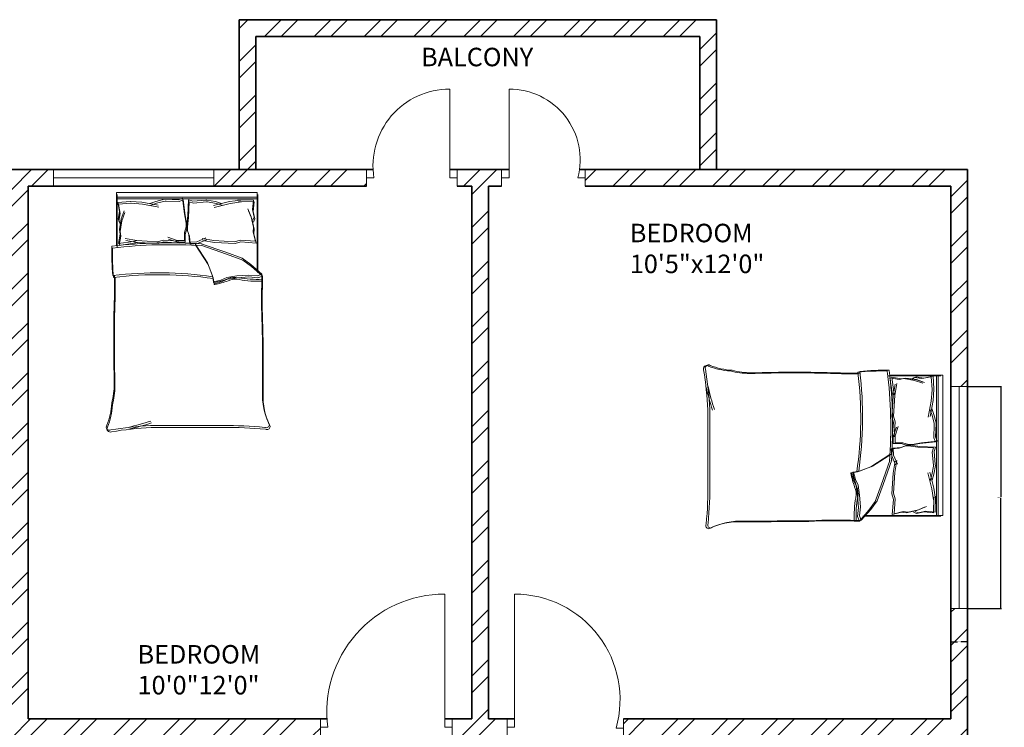
# Model space of a CAD drawing. Units: inches. Extents: x 1944 to 3454, y 1352 to 3055.
# Tile 9 of 17: x 2314 to 2580, y 2031 to 2223. Entities that reach past the tile are written whole.
import ezdxf

# ---------------------------------------------------------------- set-up
doc = ezdxf.new("R2010")
doc.units = ezdxf.units.IN
for name, color, linetype, lineweight in [('A-ANNO-DIMS', 2, 'Continuous', 18), ('A-AREA-IDEN', 7, 'Continuous', 18), ('A-DOOR', 3, 'Continuous', 20), ('A-FURN', 8, 'Continuous', 13), ('A-GLAZ', 4, 'Continuous', 18), ('A-WALL', 7, 'Continuous', 35), ('A-WALL-PATT', 252, 'Continuous', 13)]:
    doc.layers.add(name, color=color, linetype=linetype, lineweight=lineweight)
doc.styles.get("Standard").update_dxf_attribs({"font": 'arial.ttf'})
doc.dimstyles.get("Standard").update_dxf_attribs({"dimtxt": 0.18, "dimasz": 0.18, "dimexe": 0.18, "dimexo": 0.0625, "dimgap": 0.09, "dimtad": 0, "dimtih": 1, "dimtoh": 1, "dimdec": 4, "dimzin": 0, "dimdsep": 46, "dimtxsty": 'Standard', "dimcen": 0.09, "dimadec": 0, "dimazin": 0, "dimtfac": 1, "dimtdec": 4, "dimtofl": 0, "dimtmove": 0, "dimatfit": 3, "dimfxl": 1, "dimtolj": 1, "dimtzin": 0, "dimarcsym": 0})

# ---------------------------------------------------------------- blocks, each defined once
blk = doc.blocks.new('BED-WITH-PILLOWS-01')
for p, q in [((0, 40.75), (21.15, 40.75)), ((0, 40.75), (21.15, 40.75)), ((0, 2.76), (0, 40.75)), ((0.51, 40.93), (21.66, 40.93)), ((0.51, 40.93), (21.66, 40.93)), ((1.22, 2.76), (1.22, 40.75)), ((1.22, 2.76), (1.22, 40.75)), ((1.73, 2.94), (1.73, 40.93)), ((1.73, 2.94), (1.73, 40.93)), ((2.54, 40.01), (2.46, 35.72)), ((2.54, 40.01), (2.46, 35.72)), ((2.54, 40.01), (5.09, 39.71)), ((2.54, 40.01), (5.09, 39.71)), ((4.58, 39.53), (6.63, 40.01)), ((4.58, 39.53), (6.63, 40.01)), ((5.09, 39.71), (7.14, 40.19)), ((5.09, 39.71), (7.14, 40.19)), ((6.63, 40.01), (7.46, 39.6)), ((6.63, 40.01), (7.46, 39.6)), ((9.91, 40.01), (7.07, 39.38)), ((9.91, 40.01), (7.07, 39.38)), ((7.14, 40.19), (7.97, 39.78)), ((7.14, 40.19), (7.97, 39.78)), ((11.19, 39.86), (9.91, 40.01)), ((11.19, 39.86), (9.91, 40.01)), ((13.17, 40.3), (10.68, 39.68)), ((13.17, 40.3), (10.68, 39.68)), ((13.68, 40.48), (11.19, 39.86)), ((13.68, 40.48), (11.19, 39.86)), ((12.85, 36.22), (13.17, 40.3)), ((12.85, 36.22), (13.17, 40.3)), ((13.36, 36.4), (13.68, 40.48)), ((13.36, 36.4), (13.68, 40.48)), ((22.05, 42.02), (19.47, 39.08)), ((22.05, 42.02), (19.47, 39.08)), ((22.56, 42.21), (19.98, 39.26)), ((22.56, 42.21), (19.98, 39.26)), ((23.44, 42.09), (22.05, 42.02, 3.08)), ((23.44, 42.09), (22.05, 42.02, 3.08)), ((22.55, 40.8), (22.05, 42.02)), ((22.55, 40.8), (22.05, 42.02)), ((22.3, 38.34), (22.55, 40.8)), ((22.3, 38.34), (22.55, 40.8)), ((23.95, 42.27), (22.56, 42.21, 3.08)), ((23.95, 42.27), (22.56, 42.21, 3.08)), ((23.05, 40.98), (22.56, 42.21)), ((23.05, 40.98), (22.56, 42.21)), ((22.81, 38.52), (23.05, 40.98)), ((22.81, 38.52), (23.05, 40.98)), ((2.03, 39.83), (1.96, 35.54)), ((2.03, 39.83), (1.96, 35.54)), ((2.03, 39.83), (4.58, 39.53)), ((2.03, 39.83), (4.58, 39.53)), ((6.56, 39.2), (4.43, 38.26)), ((6.56, 39.2), (4.43, 38.26)), ((7.07, 39.38), (4.94, 38.44)), ((7.07, 39.38), (4.94, 38.44)), ((9.4, 39.83), (6.56, 39.2)), ((9.4, 39.83), (6.56, 39.2)), ((10.68, 39.68), (9.4, 39.83)), ((10.68, 39.68), (9.4, 39.83)), ((19.47, 39.08), (17.75, 36.74)), ((19.47, 39.08), (17.75, 36.74)), ((19.98, 39.26), (18.26, 36.92)), ((19.98, 39.26), (18.26, 36.92)), ((22.55, 35.26), (22.3, 38.34)), ((22.55, 35.26), (22.3, 38.34)), ((23.05, 35.44), (22.81, 38.52)), ((23.05, 35.44), (22.81, 38.52)), ((1.96, 35.54), (2.02, 36.34)), ((1.96, 35.54), (2.02, 36.34)), ((2.02, 36.34), (2.44, 33.32)), ((2.02, 36.34), (2.44, 33.32)), ((2.46, 35.72), (2.53, 36.52)), ((2.46, 35.72), (2.53, 36.52)), ((2.53, 36.52), (2.95, 33.5)), ((2.53, 36.52), (2.95, 33.5)), ((13.3, 34.66), (12.85, 36.22)), ((13.3, 34.66), (12.85, 36.22)), ((12.95, 29.09), (13.3, 34.66)), ((12.95, 29.09), (13.3, 34.66)), ((13.8, 34.84), (13.36, 36.4)), ((13.8, 34.84), (13.36, 36.4)), ((13.46, 29.27), (13.8, 34.84)), ((13.46, 29.27), (13.8, 34.84)), ((17.75, 36.74), (16.15, 32.31)), ((17.75, 36.74), (16.15, 32.31)), ((18.26, 36.92), (16.66, 32.49)), ((18.26, 36.92), (16.66, 32.49)), ((22.92, 32.55), (22.55, 35.26)), ((22.92, 32.55), (22.55, 35.26)), ((23.42, 32.74), (23.05, 35.44)), ((23.42, 32.74), (23.05, 35.44)), ((2.44, 33.32), (3.51, 29.01)), ((2.44, 33.32), (3.51, 29.01)), ((2.95, 33.5), (4.02, 29.19)), ((2.95, 33.5), (4.02, 29.19)), ((16.15, 32.31), (13.82, 25.68)), ((16.15, 32.31), (13.82, 25.68)), ((16.66, 32.49), (14.33, 25.86)), ((16.66, 32.49), (14.33, 25.86)), ((23.65, 30.95), (22.92, 32.55)), ((23.65, 30.95), (22.92, 32.55)), ((24.16, 31.13), (23.42, 32.74)), ((24.16, 31.13), (23.42, 32.74)), ((2.45, 29.52), (2.02, 27.19)), ((2.45, 29.52), (2.02, 27.19)), ((2.92, 31.16), (2.45, 29.52)), ((2.92, 31.16), (2.45, 29.52)), ((2.95, 29.7), (2.52, 27.37)), ((2.95, 29.7), (2.52, 27.37)), ((3.43, 31.34), (2.95, 29.7)), ((3.43, 31.34), (2.95, 29.7)), ((24.15, 28.98), (23.65, 30.95)), ((24.15, 28.98), (23.65, 30.95)), ((24.65, 29.17), (24.16, 31.13)), ((24.65, 29.16), (24.16, 31.13)), ((62.99, 11.97), (62.99, 31.54)), ((62.99, 11.97), (62.99, 31.54)), ((63.5, 12.16), (63.5, 31.72)), ((63.5, 12.15), (63.5, 31.72)), ((2.02, 27.19), (2.03, 26.93)), ((2.02, 27.19), (2.03, 26.93)), ((2.03, 26.93), (2.37, 23.41)), ((2.03, 26.93), (2.37, 23.41)), ((2.52, 27.37), (2.54, 27.12)), ((2.52, 27.37), (2.54, 27.11)), ((2.54, 27.12), (2.88, 23.6)), ((2.54, 27.11), (2.88, 23.6)), ((13.31, 24.44), (12.28, 26.88)), ((13.31, 24.44), (12.28, 26.88)), ((12.42, 25.88), (12.95, 29.09)), ((12.42, 25.88), (12.95, 29.09)), ((13.81, 24.62), (12.79, 27.07)), ((13.81, 24.62), (12.79, 27.06)), ((12.93, 26.07), (13.46, 29.27)), ((12.93, 26.07), (13.46, 29.27)), ((13.82, 24.05), (18.98, 27.38)), ((13.82, 24.05), (18.98, 27.38)), ((14.33, 24.23), (19.49, 27.56)), ((14.33, 24.23), (19.49, 27.56)), ((18.98, 27.38), (22.55, 28.74)), ((18.98, 27.38), (22.55, 28.74)), ((19.49, 27.56), (23.05, 28.92)), ((19.49, 27.56), (23.05, 28.92)), ((22.55, 28.74), (24.15, 28.98)), ((22.55, 28.74), (24.15, 28.98)), ((23.05, 28.92), (24.65, 29.17)), ((23.05, 28.92), (24.65, 29.16)), ((13.43, 22.49), (13.31, 24.44)), ((13.43, 22.49), (13.31, 24.44)), ((13.94, 22.67), (13.81, 24.62)), ((13.94, 22.67), (13.81, 24.62)), ((2.37, 23.41), (1.98, 22.24)), ((2.37, 23.41), (1.98, 22.24)), ((1.98, 22.24), (6.25, 22.04)), ((1.98, 22.24), (6.25, 22.04)), ((2.88, 23.6), (2.49, 22.42)), ((2.88, 23.6), (2.49, 22.42)), ((2.49, 22.42), (6.76, 22.23)), ((2.49, 22.42), (6.76, 22.23)), ((5.74, 21.11), (8.27, 21.57)), ((5.74, 21.11), (8.27, 21.57)), ((6.25, 22.04), (8.81, 21.74)), ((6.25, 22.04), (8.81, 21.74)), ((6.25, 21.29), (8.78, 21.75)), ((6.25, 21.29), (8.78, 21.75)), ((6.76, 22.23), (9.31, 21.93)), ((6.76, 22.23), (9.31, 21.93)), ((8.27, 21.57), (9.3, 21.57)), ((8.27, 21.57), (9.3, 21.57)), ((8.78, 21.75), (9.81, 21.75)), ((8.78, 21.75), (9.81, 21.75)), ((8.81, 21.74), (9.84, 21.81)), ((8.81, 21.74), (9.84, 21.81)), ((9.3, 21.57), (10.8, 21.11)), ((9.3, 21.57), (10.8, 21.11)), ((9.31, 21.93), (10.35, 21.99)), ((9.31, 21.93), (10.35, 21.99)), ((9.81, 21.75), (11.3, 21.29)), ((9.81, 21.75), (11.3, 21.29)), ((9.84, 21.81), (11.3, 22.36)), ((9.84, 21.81), (11.3, 22.36)), ((10.35, 21.99), (11.81, 22.54)), ((10.35, 21.99), (11.81, 22.54)), ((11.3, 22.36), (13.43, 22.49)), ((11.3, 22.36), (13.43, 22.49)), ((11.81, 22.54), (13.94, 22.67)), ((11.81, 22.54), (13.94, 22.67)), ((1.49, 20.65), (5.74, 21.11)), ((1.49, 20.65), (5.74, 21.11)), ((1.95, 19.5), (1.49, 20.65)), ((1.95, 19.5), (1.49, 20.65)), ((1.83, 15.97), (1.95, 19.5)), ((1.83, 15.97), (1.95, 19.5)), ((1.99, 20.83), (6.25, 21.29)), ((1.99, 20.83), (6.25, 21.29)), ((2.45, 19.69), (1.99, 20.83)), ((2.45, 19.69), (1.99, 20.83)), ((2.34, 16.15), (2.45, 19.69)), ((2.34, 16.15), (2.45, 19.69)), ((10.8, 21.11), (12.93, 21.11)), ((10.8, 21.11), (12.93, 21.11)), ((11.3, 21.29), (13.44, 21.29)), ((11.3, 21.29), (13.44, 21.29)), ((12.93, 19.16), (12.06, 16.66)), ((12.93, 19.16), (12.06, 16.66)), ((13.44, 19.34), (12.57, 16.84)), ((13.44, 19.34), (12.57, 16.84)), ((12.85, 15.41), (13.17, 19.49)), ((12.85, 15.41), (13.17, 19.49)), ((12.93, 21.11), (12.93, 19.16)), ((12.93, 21.11), (12.93, 19.16)), ((13.36, 15.59), (13.68, 19.67)), ((13.36, 15.59), (13.68, 19.67)), ((13.44, 21.29), (13.44, 19.34)), ((13.44, 21.29), (13.44, 19.34)), ((2.34, 15.9), (2.34, 16.15)), ((2.34, 15.9), (2.34, 16.15)), ((1.83, 15.71), (1.83, 15.97)), ((1.83, 15.71), (1.83, 15.97)), ((2.41, 13.42), (1.83, 15.71)), ((2.41, 13.42), (1.83, 15.71)), ((2.91, 13.6), (2.34, 15.9)), ((2.91, 13.6), (2.34, 15.9)), ((2.98, 11.81), (2.41, 13.42)), ((2.98, 11.81), (2.41, 13.42)), ((2.64, 9.62), (3.44, 13.99)), ((2.64, 9.62), (3.44, 13.99)), ((3.49, 11.99), (2.91, 13.6)), ((3.49, 11.99), (2.91, 13.6)), ((3.14, 9.81), (3.95, 14.17)), ((3.14, 9.81), (3.95, 14.17)), ((13.3, 13.85), (12.85, 15.41)), ((13.3, 13.85), (12.85, 15.41)), ((12.95, 8.28), (13.3, 13.85)), ((12.95, 8.28), (13.3, 13.85)), ((13.8, 14.03), (13.36, 15.59)), ((13.8, 14.03), (13.36, 15.59)), ((13.46, 8.46), (13.8, 14.03)), ((13.46, 8.46), (13.8, 14.03)), ((2.41, 6.59), (2.64, 9.62)), ((2.41, 6.59), (2.64, 9.62)), ((2.91, 6.77), (3.14, 9.81)), ((2.91, 6.77), (3.14, 9.81)), ((12.42, 5.07), (12.95, 8.28)), ((12.42, 5.07), (12.95, 8.28)), ((12.93, 5.25), (13.46, 8.46)), ((12.93, 5.25), (13.46, 8.46)), ((12.95, 8.28), (13.21, 7.38)), ((12.95, 8.28), (13.21, 7.38)), ((13.46, 8.46), (13.72, 7.56)), ((13.46, 8.46), (13.72, 7.56)), ((2.39, 6.5), (2.41, 6.59)), ((2.39, 6.5), (2.41, 6.59)), ((2.65, 3.1), (2.39, 6.5)), ((2.65, 3.1), (2.39, 6.5)), ((2.9, 6.68), (2.91, 6.77)), ((2.9, 6.68), (2.91, 6.77)), ((3.16, 3.28), (2.9, 6.68)), ((3.16, 3.28), (2.9, 6.68)), ((13.21, 7.38), (13.78, 3.33)), ((13.21, 7.38), (13.78, 3.33)), ((13.72, 7.56), (14.29, 3.51)), ((13.72, 7.56), (14.29, 3.51)), ((14.4, 2.76), (0, 2.76)), ((14.4, 2.76), (0, 2.76)), ((14.9, 2.94), (0.51, 2.94)), ((14.9, 2.94), (0.51, 2.94)), ((2.64, 3.1), (5.16, 3.56)), ((2.64, 3.1), (5.16, 3.56)), ((3.14, 3.28), (5.67, 3.74)), ((3.14, 3.28), (5.67, 3.74)), ((7.12, 4.02), (4.93, 4.82)), ((7.12, 4.01), (4.93, 4.82)), ((5.16, 3.56), (7.23, 3.21)), ((5.16, 3.56), (7.23, 3.21)), ((7.63, 4.2), (5.44, 5)), ((7.63, 4.2), (5.44, 5)), ((5.67, 3.74), (7.74, 3.39)), ((5.67, 3.74), (7.74, 3.39)), ((9.99, 3.56), (7.12, 4.02)), ((9.99, 3.56), (7.12, 4.01)), ((7.23, 3.21), (8.04, 3.67)), ((7.23, 3.21), (8.04, 3.67)), ((10.5, 3.74), (7.63, 4.2)), ((10.5, 3.74), (7.63, 4.2)), ((7.74, 3.39), (8.55, 3.85)), ((7.74, 3.39), (8.55, 3.85)), ((11.26, 3.79), (9.99, 3.56)), ((11.26, 3.79), (9.99, 3.56)), ((11.76, 3.97), (10.5, 3.74)), ((11.76, 3.97), (10.5, 3.74)), ((13.78, 3.33), (11.26, 3.79)), ((13.78, 3.33), (11.26, 3.79)), ((14.29, 3.51), (11.76, 3.97)), ((14.29, 3.51), (11.76, 3.97))]:
    blk.add_line(p, q)
for centre, radius, start, end in [((54.58, 60.54), 18.33, 267.4714, 296.4681), ((54.58, 60.54), 18.33, 267.4714, 296.4681), ((55.09, 60.72), 18.33, 267.4714, 296.4681), ((55.09, 60.72), 18.33, 267.4714, 296.4681), ((62.69, 43.25), 0.876, 332.6588, 86.02), ((62.69, 43.25), 0.876, 332.6588, 86.02), ((168.74, 32.71), 105.75, 174.4998, 180.6351), ((168.74, 32.71), 105.75, 174.4998, 180.6351), ((63.2, 43.43), 0.876, 332.6588, 86.02), ((63.2, 43.43), 0.876, 332.6588, 86.02), ((169.24, 32.89), 105.75, 174.4998, 180.6351), ((169.24, 32.89), 105.75, 174.4998, 180.6351), ((-5.29, 40.8), 28.76, 349.8763, 2.5657), ((-5.29, 40.8), 28.76, 349.8763, 2.5657), ((28.87, 144.88), 102.94, 266.9791, 273.8365), ((28.87, 144.88), 102.94, 266.9791, 273.8365), ((-4.78, 40.98), 28.76, 349.8763, 2.5657), ((-4.78, 40.98), 28.76, 349.8763, 2.5657), ((29.37, 145.06), 102.94, 266.9791, 273.8365), ((29.37, 145.06), 102.94, 266.9791, 273.8365), ((53.91, -3583.94), 3626.16, 90.00217, 90.28689), ((53.91, -3583.94), 3626.16, 90.00217, 90.28689), ((54.42, -3583.76), 3626.16, 90.00217, 90.28689), ((54.42, -3583.76), 3626.16, 90.00217, 90.28689), ((27.87, 34.77), 4.95, 168.6608, 203.7384), ((27.87, 34.77), 4.95, 168.6608, 203.7384), ((28.38, 34.95), 4.95, 168.6608, 203.7384), ((28.38, 34.95), 4.95, 168.6608, 203.7384), ((1.18, 24.76), 23.57, 10.6617, 19.8806), ((1.18, 24.76), 23.57, 10.6617, 19.8806), ((1.69, 24.95), 23.57, 10.6617, 19.8806), ((1.69, 24.94), 23.57, 10.6617, 19.8806), ((24.7, 29.3), 0.147, 250.2464, 1.1377), ((24.7, 29.3), 0.147, 250.2464, 1.1377), ((124.25, 14.11), 102.56, 171.7845, 186.9006), ((124.25, 14.11), 102.56, 171.7845, 186.9006), ((124.76, 14.3), 102.56, 171.7845, 186.9006), ((124.76, 14.3), 102.56, 171.7845, 186.9006), ((24.2, 29.12), 0.147, 250.2464, 1.1377), ((24.2, 29.12), 0.147, 250.2464, 1.1377), ((144.71, 16.98), 131.13, 176.0865, 186.7821), ((144.71, 16.98), 131.13, 176.0865, 186.7821), ((145.22, 17.16), 131.13, 176.0865, 186.7821), ((145.22, 17.16), 131.13, 176.0865, 186.7821), ((-18.85, -13.69), 84.62, 13.3832, 17.7053), ((-18.85, -13.69), 84.62, 13.3832, 17.7053), ((-18.34, -13.51), 84.62, 13.3832, 17.7053), ((-18.34, -13.51), 84.62, 13.3832, 17.7053), ((159.64, 17.03), 96.78, 182.9958, 189.4091), ((159.64, 17.03), 96.78, 182.9958, 189.4091), ((160.15, 17.21), 96.78, 182.9958, 189.4091), ((160.15, 17.21), 96.78, 182.9958, 189.4091), ((15.97, 67.69), 66.22, 268.7218, 275.604), ((15.97, 67.69), 66.22, 268.7218, 275.604), ((16.48, 67.88), 66.22, 268.7218, 275.604), ((16.48, 67.88), 66.22, 268.7218, 275.604), ((24.78, -132.99), 135.22, 88.4762, 91.0082), ((24.78, -132.99), 135.22, 88.4762, 91.0082), ((25.29, -132.81), 135.22, 88.4762, 91.0082), ((25.29, -132.81), 135.22, 88.4762, 91.0082), ((40.23, 385.38), 383.38, 268.2277, 271.7185), ((40.23, 385.38), 383.38, 268.2277, 271.7185), ((40.74, 385.56), 383.38, 268.2277, 271.7185), ((40.74, 385.56), 383.38, 268.2277, 271.7185), ((51.28, -21.38), 23.56, 76.0648, 88.9113), ((51.28, -21.38), 23.56, 76.0648, 88.9113), ((51.79, -21.2), 23.56, 76.0648, 88.9113), ((51.79, -21.2), 23.56, 76.0648, 88.9113), ((55.86, -17.22), 18.73, 67.9751, 86.652), ((55.86, -17.22), 18.73, 67.9751, 86.652), ((56.37, -17.04), 18.73, 67.9751, 86.652), ((56.37, -17.04), 18.73, 67.9751, 86.652), ((63.37, 0.86), 0.866, 236.1736, 23.4781), ((63.37, 0.86), 0.866, 236.1736, 23.4781), ((63.87, 1.05), 0.866, 236.1736, 23.4781), ((63.87, 1.05), 0.866, 236.1736, 23.4781)]:
    blk.add_arc(centre, radius, start, end)
blk = doc.blocks.new('DOOR-SWING-36IN-01')
for p, q in [((33.61, 2.25), (33.61, 38.25)), ((0, 4.5), (0, 0)), ((0, 0), (0, 4.5)), ((0, 4.5), (0, 2.25)), ((35.61, 4.5), (35.61, 0)), ((0, 2.25), (2, 2.25)), ((35.61, 2.25), (33.61, 2.25)), ((35.61, 0), (35.61, 2.25))]:
    blk.add_line(p, q)
blk.add_arc((33.61, 6.37), 31.88, 90, 187.4328)
blk = doc.blocks.new('DOOR-SWING-36IN-02')
for p, q in [((2, 2.65), (2, 38.65)), ((0, 4.9), (0, 0.4)), ((31.45, 4.9), (31.45, 0)), ((0, 0.4), (0, 2.65)), ((0, 2.65), (2, 2.65)), ((31.45, 2.45), (29.45, 2.45))]:
    blk.add_line(p, q)
blk.add_arc((2, 10.14), 28.51, 344.3464, 90)
blk = doc.blocks.new('DOOR-SWING-24IN-03')
for p, q in [((22.49, 2.25), (22.49, 26.25)), ((0, 4.5), (0, 0)), ((24.49, 0), (24.49, 4.5)), ((24.49, 4.5), (24.49, 2.25)), ((0, 0), (0, 2.25)), ((0, 2.25), (2, 2.25)), ((24.49, 2.25), (22.49, 2.25))]:
    blk.add_line(p, q)
blk.add_arc((22.49, 5.5), 20.75, 90, 189.0124)
blk = doc.blocks.new('DOOR-SWING-24IN-04')
for p, q in [((2, 2.25), (2, 26.25)), ((0, 0), (0, 4.5)), ((0, 4.5), (0, 2.25)), ((22.61, 4.5), (22.61, 0)), ((0, 2.25), (2, 2.25)), ((22.61, 2.25), (20.61, 2.25)), ((22.61, 0), (22.61, 2.25))]:
    blk.add_line(p, q)
blk.add_arc((2.1, 7.11), 19.14, 345.2922, 90.304)
blk = doc.blocks.new('WINDOW-PLAN-60.00IN-02')
for p, q in [((2.25, 60), (0, 60)), ((0, 60), (4.5, 60)), ((2.25, 0), (2.25, 60)), ((0, 0), (4.5, 0)), ((4.5, 0), (2.25, 0))]:
    blk.add_line(p, q)
blk = doc.blocks.new('WINDOW-PLAN-43.38IN-01')
for p, q in [((0, 0), (0, 4.5)), ((0, 4.5), (0, 2.25)), ((43.38, 2.25), (43.38, 4.5)), ((43.38, 4.5), (43.38, 0)), ((0, 2.25), (43.38, 2.25))]:
    blk.add_line(p, q)
blk = doc.blocks.new('*D80')
at = {"layer": 'A-ANNO-DIMS', "color": 0, "lineweight": -2, "transparency": 16777216}
for p, q in [((2569.88, 2123.45), (2579, 2123.45)), ((2578.82, 2123.27), (2578.82, 2093.64)), ((2578.82, 2063.63), (2578.82, 2093.27)), ((2569.88, 2063.45), (2579, 2063.45))]:
    blk.add_line(p, q, dxfattribs=at)
at = {"layer": 'A-ANNO-DIMS', "color": 0, "transparency": 16777216}
for points in [[(2578.79, 2123.27), (2578.85, 2123.27), (2578.82, 2123.45)], [(2578.79, 2063.63), (2578.85, 2063.63), (2578.82, 2063.45)]]:
    blk.add_solid(points, dxfattribs=at)
at = {"layer": 'Defpoints', "color": 0, "transparency": 16777216}
for p in [(2569.82, 2123.45), (2578.82, 2123.45), (2569.82, 2063.45)]:
    blk.add_point(p, dxfattribs=at)
at = {"layer": 'A-ANNO-DIMS', "color": 0, "transparency": 16777216, "insert": (2578.82, 2093.45), "char_height": 0.18, "attachment_point": 5}
blk.add_mtext('\\A1;WINDOW 60 TYP.', dxfattribs=at)
blk = doc.blocks.new('*D81')
at = {"layer": 'A-ANNO-DIMS', "color": 0, "lineweight": -2, "transparency": 16777216}
for p, q in [((2565.32, 2063.39), (2565.32, 2054.27)), ((2569.82, 2063.39), (2569.82, 2054.27)), ((2565.5, 2054.45), (2567.11, 2054.45)), ((2569.64, 2054.45), (2568.03, 2054.45))]:
    blk.add_line(p, q, dxfattribs=at)
at = {"layer": 'A-ANNO-DIMS', "color": 0, "transparency": 16777216}
for points in [[(2565.5, 2054.48), (2565.5, 2054.42), (2565.32, 2054.45)], [(2569.64, 2054.48), (2569.64, 2054.42), (2569.82, 2054.45)]]:
    blk.add_solid(points, dxfattribs=at)
at = {"layer": 'Defpoints', "color": 0, "transparency": 16777216}
for p in [(2565.32, 2063.45), (2569.82, 2063.45), (2569.82, 2054.45)]:
    blk.add_point(p, dxfattribs=at)
at = {"layer": 'A-ANNO-DIMS', "color": 0, "transparency": 16777216, "insert": (2567.57, 2054.45), "char_height": 0.18, "attachment_point": 5}
blk.add_mtext('\\A1;5 TYP.', dxfattribs=at)

msp = doc.modelspace()

# ---------------------------------------------------------------- hatches: boundary and pattern name
at = {"layer": 'A-WALL-PATT'}
h = msp.add_hatch(dxfattribs=at)
h.set_pattern_fill('ANSI32', color=256)
h.paths.add_polyline_path([(2061.822, 2177.596), (2158.181, 2177.596), (2158.181, 2179.846), (2158.181, 2182.096), (2057.322, 2182.096), (2057.322, 2123.452), (2061.822, 2123.452)])
h.paths.add_polyline_path([(2258.993, 2179.846), (2258.993, 2182.096), (2218.838, 2182.096), (2218.838, 2177.596), (2258.993, 2177.596)])
h.paths.add_polyline_path([(2315.822, 2177.596), (2322.722, 2177.596), (2322.722, 2182.096), (2303.186, 2182.096), (2303.186, 2177.596), (2311.322, 2177.596), (2311.322, 2033.596), (2231.355, 2033.596), (2231.355, 2029.096), (2311.322, 2029.096), (2311.322, 1904.596), (2307.941, 1904.596), (2307.941, 1900.096), (2319.277, 1900.096), (2319.277, 1902.346), (2319.277, 1904.596), (2315.822, 1904.596), (2315.822, 2029.096), (2394.855, 2029.096), (2394.855, 2033.596), (2315.822, 2033.596)])
h.paths.add_polyline_path([(2407.334, 2182.096), (2366.1, 2182.096), (2366.1, 2177.596), (2407.334, 2177.596), (2407.334, 2179.846)])
h.paths.add_polyline_path([(2440.322, 2177.596), (2443.866, 2177.596), (2443.866, 2182.096), (2431.827, 2182.096), (2431.827, 2179.846), (2431.827, 2177.596), (2435.822, 2177.596), (2435.822, 2033.596), (2430.464, 2033.596), (2430.464, 2029.096), (2445.372, 2029.096), (2445.372, 2031.346), (2445.372, 2033.596), (2440.322, 2033.596)])
h.paths.add_polyline_path([(2569.822, 2182.096), (2466.481, 2182.096), (2466.481, 2177.596), (2565.322, 2177.596), (2565.322, 2123.452), (2569.822, 2123.452)])
h.paths.add_polyline_path([(2569.822, 2063.452), (2567.572, 2063.452), (2565.322, 2063.452), (2565.322, 2033.596), (2478.08, 2033.596), (2476.822, 2033.596), (2476.822, 2028.698), (2476.822, 2020.069), (2481.322, 2020.069), (2481.322, 2029.096), (2565.322, 2029.096), (2565.322, 2014.5), (2569.822, 2014.5)])
h.paths.add_polyline_path([(2569.822, 1978.5), (2565.322, 1978.5), (2565.322, 1957.096), (2481.322, 1957.096), (2481.322, 1990.369), (2476.822, 1990.369), (2476.822, 1957.096), (2476.822, 1952.596), (2476.822, 1947.471), (2481.322, 1947.471), (2481.322, 1952.596), (2565.322, 1952.596), (2565.322, 1943.2), (2569.822, 1943.2)])
h.paths.add_polyline_path([(2569.822, 1919.2), (2565.322, 1919.2), (2565.322, 1904.596), (2481.322, 1904.596), (2481.322, 1928.596), (2476.822, 1928.596), (2476.822, 1904.596), (2350.518, 1904.596), (2350.518, 1900.096), (2476.822, 1900.096), (2565.322, 1900.096), (2565.322, 1895.596), (2565.322, 1887.047), (2569.822, 1887.047)])
h.paths.add_polyline_path([(2280.492, 1904.596), (2150.322, 1904.596), (2150.322, 1926.68), (2148.072, 1926.68), (2145.822, 1926.68), (2145.822, 1904.596), (2061.822, 1904.596), (2061.822, 1914.977), (2059.572, 1914.977), (2057.322, 1914.977), (2057.322, 1887.362), (2061.822, 1887.362), (2061.822, 1900.096), (2150.322, 1900.096), (2280.492, 1900.096), (2280.492, 1902.346)])
h.paths.add_polyline_path([(2150.322, 1957.096), (2150.322, 1986.22), (2145.822, 1986.22), (2145.822, 1957.096), (2061.822, 1957.096), (2061.822, 1975.678), (2057.322, 1975.678), (2057.322, 1938.977), (2061.822, 1938.977), (2061.822, 1952.596), (2145.822, 1952.596), (2145.822, 1947.985), (2150.322, 1947.985), (2150.322, 1952.596)])
h.paths.add_polyline_path([(2061.822, 2063.452), (2057.322, 2063.452), (2057.322, 2011.678), (2061.822, 2011.678), (2061.822, 2029.096), (2145.288, 2029.096), (2145.822, 2029.096), (2145.822, 2019.118), (2150.322, 2019.118), (2150.322, 2029.096), (2150.322, 2033.596), (2147.022, 2033.596), (2061.822, 2033.596)])
h.paths.add_polyline_path([(2061.822, 1835.596), (2133.822, 1835.596), (2133.822, 1794.415), (2138.322, 1794.415), (2138.322, 1835.596), (2231.726, 1835.596), (2231.726, 1840.096), (2061.822, 1840.096), (2061.822, 1851.362), (2057.322, 1851.362), (2057.322, 1810.528), (2061.822, 1810.528)])
h.paths.add_polyline_path([(2061.822, 1774.528), (2059.572, 1774.528), (2057.322, 1774.528), (2057.322, 1723.746), (2061.822, 1723.746), (2061.822, 1735.096), (2133.822, 1735.096), (2133.822, 1731.415), (2138.322, 1731.415), (2138.322, 1759.737), (2133.822, 1759.737), (2133.822, 1739.596), (2061.822, 1739.596)])
h.paths.add_polyline_path([(2061.822, 1678.596), (2147.597, 1678.596), (2147.597, 1680.846), (2147.597, 1683.096), (2138.322, 1683.096), (2138.322, 1710.66), (2136.072, 1710.66), (2133.822, 1710.66), (2133.822, 1683.096), (2061.822, 1683.096), (2061.822, 1699.746), (2057.322, 1699.746), (2057.322, 1645.751), (2061.822, 1645.751)])
h.paths.add_polyline_path([(2061.822, 1585.751), (2057.322, 1585.751), (2057.322, 1530.096), (2158.703, 1530.096), (2158.703, 1534.596), (2061.822, 1534.596)])
h.paths.add_polyline_path([(2191.322, 1678.596), (2195.889, 1678.596), (2195.889, 1683.096), (2181.763, 1683.096), (2181.763, 1680.846), (2181.763, 1678.596), (2186.822, 1678.596), (2186.822, 1534.596), (2181.354, 1534.596), (2181.354, 1530.096), (2196.54, 1530.096), (2196.54, 1532.346), (2196.54, 1534.596), (2191.322, 1534.596)])
h.paths.add_polyline_path([(2315.822, 1678.596), (2402.014, 1678.596), (2402.014, 1683.096), (2355.822, 1683.096), (2355.822, 1835.596), (2360.838, 1835.596), (2360.838, 1840.096), (2351.322, 1840.096), (2351.322, 1683.096), (2273.322, 1683.096), (2273.322, 1840.096), (2263.134, 1840.096), (2263.134, 1837.846), (2263.134, 1835.596), (2268.822, 1835.596), (2268.822, 1683.096), (2227.793, 1683.096), (2227.793, 1678.596), (2311.322, 1678.596), (2311.322, 1534.596), (2302.384, 1534.596), (2302.384, 1530.096), (2324.521, 1530.096), (2324.521, 1532.346), (2324.521, 1534.596), (2315.822, 1534.596)])
h.paths.add_polyline_path([(2440.322, 1678.596), (2443.656, 1678.596), (2443.656, 1683.096), (2432.614, 1683.096), (2432.614, 1680.846), (2432.614, 1678.596), (2435.822, 1678.596), (2435.822, 1534.596), (2440.322, 1534.596)])
h.paths.add_polyline_path([(2409.913, 1534.596), (2369.033, 1534.596), (2369.033, 1530.096), (2409.913, 1530.096)])
h.paths.add_polyline_path([(2259.529, 1532.346), (2259.529, 1534.596), (2218.889, 1534.596), (2218.889, 1532.346), (2218.889, 1530.096), (2259.529, 1530.096)])
h.paths.add_polyline_path([(2569.822, 1584.389), (2567.572, 1584.389), (2565.322, 1584.389), (2565.322, 1534.596), (2465.892, 1534.596), (2465.892, 1530.096), (2569.822, 1530.096)])
h.paths.add_polyline_path([(2505.567, 1530.096), (2501.067, 1530.096), (2501.067, 1494.096), (2381.067, 1494.096), (2381.067, 1530.096), (2376.567, 1530.096), (2376.567, 1489.596), (2381.067, 1489.596), (2505.567, 1489.596), (2505.567, 1494.096)])
h.paths.add_polyline_path([(2127.673, 1530.096), (2123.173, 1530.096), (2123.173, 1489.596), (2127.673, 1489.596), (2252.173, 1489.596), (2252.173, 1494.096), (2252.173, 1530.096), (2247.673, 1530.096), (2247.673, 1494.096), (2127.673, 1494.096)])
h.paths.add_polyline_path([(2251.167, 2222.596), (2126.667, 2222.596), (2122.167, 2222.596), (2122.167, 2182.096), (2126.667, 2182.096), (2126.667, 2218.096), (2210.667, 2218.096), (2234.667, 2218.096), (2246.667, 2218.096), (2246.667, 2182.096), (2251.167, 2182.096), (2251.167, 2218.096)])
h.paths.add_polyline_path([(2501.916, 2222.596), (2497.416, 2222.596), (2372.916, 2222.596), (2372.916, 2218.096), (2372.916, 2182.096), (2377.416, 2182.096), (2377.416, 2218.096), (2497.416, 2218.096), (2497.416, 2182.096), (2501.916, 2182.096)])
h.paths.add_polyline_path([(2569.822, 1700.442), (2565.322, 1700.442), (2565.322, 1683.096), (2493.322, 1683.096), (2493.322, 1709.096), (2488.822, 1709.096), (2488.822, 1683.096), (2475.416, 1683.096), (2475.416, 1680.846), (2475.416, 1678.596), (2488.822, 1678.596), (2565.322, 1678.596), (2565.322, 1644.389), (2569.822, 1644.389)])
h.paths.add_polyline_path([(2569.822, 1773.506), (2565.322, 1773.506), (2565.322, 1739.596), (2493.322, 1739.596), (2493.322, 1754.002), (2488.822, 1754.002), (2488.822, 1729.846), (2491.072, 1729.846), (2493.322, 1729.846), (2493.322, 1735.096), (2565.322, 1735.096), (2565.322, 1724.442), (2569.822, 1724.442)])
h.paths.add_polyline_path([(2569.822, 1851.047), (2567.572, 1851.047), (2565.322, 1851.047), (2565.322, 1840.096), (2395.039, 1840.096), (2395.039, 1837.846), (2395.039, 1835.596), (2488.822, 1835.596), (2488.822, 1798.423), (2493.322, 1798.423), (2493.322, 1835.596), (2565.322, 1835.596), (2565.322, 1809.506), (2569.822, 1809.506)])
h.paths.add_polyline_path([(2347.275, 1955.576), (2414.024, 1955.576), (2414.024, 1974.234), (2347.275, 1974.234)], flags=9)
h.paths.add_polyline_path([(2509.756, 1990.497), (2542.915, 1990.497), (2542.915, 2009.154), (2509.756, 2009.154)], flags=9)

# ---------------------------------------------------------------- linework, layer by layer
at = {"layer": 'A-WALL'}
for p, q in [((2372.916, 2218.096), (2372.916, 2222.596)), ((2372.916, 2222.596), (2497.416, 2222.596)), ((2497.416, 2222.596), (2501.916, 2222.596)), ((2501.916, 2222.596), (2501.916, 2182.096)), ((2372.916, 2182.096), (2372.916, 2218.096)), ((2377.416, 2182.096), (2377.416, 2218.096)), ((2377.416, 2218.096), (2497.416, 2218.096)), ((2497.416, 2218.096), (2497.416, 2182.096)), ((2217.22, 2182.096), (2409.102, 2182.096)), ((2377.416, 2182.096), (2372.916, 2182.096)), ((2429.827, 2182.096), (2445.866, 2182.096)), ((2464.929, 2182.096), (2569.822, 2182.096)), ((2569.822, 2182.096), (2569.822, 1530.096)), ((2315.822, 2177.596), (2315.822, 2033.596)), ((2315.822, 2177.596), (2407.334, 2177.596)), ((2431.827, 2177.596), (2435.822, 2177.596)), ((2435.822, 2177.596), (2435.822, 2033.596)), ((2440.322, 2177.596), (2440.322, 2033.596)), ((2440.322, 2177.596), (2443.866, 2177.596)), ((2466.481, 2177.596), (2565.322, 2177.596)), ((2565.322, 2177.596), (2565.322, 2033.596)), ((2315.822, 2033.596), (2396.643, 2033.596)), ((2428.464, 2033.596), (2435.822, 2033.596)), ((2440.322, 2033.596), (2447.372, 2033.596)), ((2478.08, 2033.596), (2476.822, 2033.596)), ((2478.08, 2033.596), (2565.322, 2033.596))]:
    msp.add_line(p, q, dxfattribs=at)

# ---------------------------------------------------------------- block references
at = {"layer": 'A-DOOR'}
for name, p in [('DOOR-SWING-24IN-03', (2407.334, 2177.596)), ('DOOR-SWING-24IN-04', (2443.866, 2177.596)), ('DOOR-SWING-36IN-01', (2394.855, 2029.096)), ('DOOR-SWING-36IN-02', (2445.372, 2028.698))]:
    msp.add_blockref(name, p, dxfattribs=at)
at = {"layer": 'A-FURN'}
for p, rotation in [((2336.98, 2175.882), 270), ((2563.141, 2129.315), 180)]:
    msp.add_blockref('BED-WITH-PILLOWS-01', p, dxfattribs=dict(at, rotation=rotation))
at = {"layer": 'A-GLAZ'}
for name, p in [('WINDOW-PLAN-43.38IN-01', (2322.722, 2177.596)), ('WINDOW-PLAN-60.00IN-02', (2565.322, 2063.452))]:
    msp.add_blockref(name, p, dxfattribs=at)

# ---------------------------------------------------------------- texts
at = {"layer": 'A-AREA-IDEN', "char_height": 5, "attachment_point": 1}
for s, width, insert in [('BALCONY', 118.50767, (2422.09, 2215.008)), ('BEDROOM\\P10\'5"x12\'0"', 132.4618, (2478.523, 2167.441)), ('BEDROOM\\P10\'0"12\'0"', 100.65001, (2345.433, 2053.576))]:
    msp.add_mtext_dynamic_manual_height_columns(s, width=width, gutter_width=12.5, heights=[0], dxfattribs=dict(at, insert=insert))

# ---------------------------------------------------------------- dimensions: what is measured, and where the dimension line sits
at = {"layer": 'A-ANNO-DIMS'}
dim = msp.add_linear_dim(base=(2578.822, 2123.452), p1=(2569.822, 2063.452), p2=(2569.822, 2123.452), angle=90, text='WINDOW <> TYP.', dimstyle='Standard', override={"dimdec": 0, "dimlfac": 1, "dimrnd": 0, "dimzin": 0, "dimdsep": 46, "dimlunit": 2}, dxfattribs=at)
dim.commit()
dim.dimension.update_dxf_attribs({"geometry": '*D80', "text_midpoint": (2578.822, 2093.452)})
dim = msp.add_linear_dim(base=(2569.821802765, 2054.452491017), p1=(2565.321802765, 2063.452491017), p2=(2569.821802765, 2063.452491017), text='<> TYP.', dimstyle='Standard', override={"dimdec": 0, "dimlfac": 1, "dimrnd": 0, "dimzin": 0, "dimdsep": 46, "dimlunit": 2}, dxfattribs=at)
dim.commit()
dim.dimension.update_dxf_attribs({"geometry": '*D81', "text_midpoint": (2567.571802765, 2054.452491017)})

doc.saveas('drawing.dxf')
